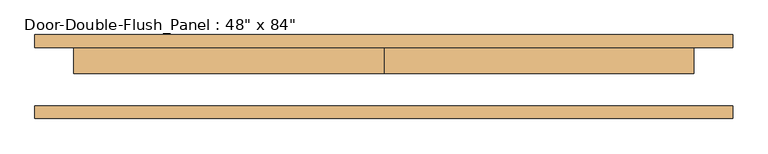
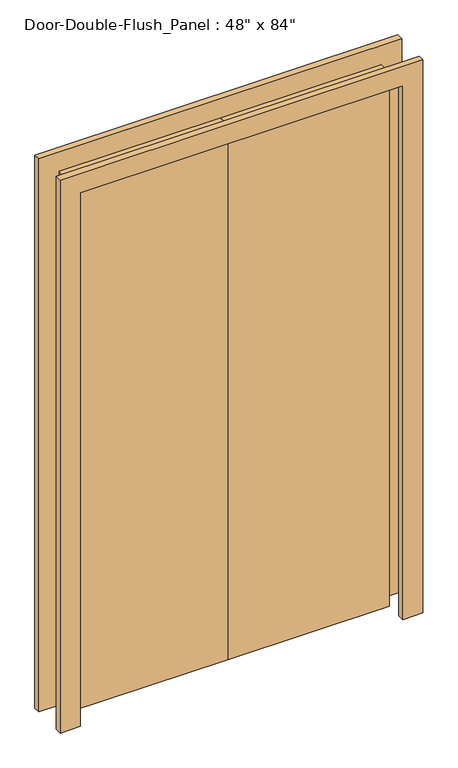
"""IFC4 building model written with IfcOpenShell, lengths in millimetres: door geometry."""

from ifc_helpers import new_model, si_unit, frame, origin, origin_with_axes, place, context, project, spatial, polyline, outline, extrude, source, transform, mapped, element, save


def door_eb8a45e1(model_context):
    return source(origin(), model_context, "Body", "SweptSolid", [
        extrude(outline(polyline([(2133.6, -609.6), (2133.6, 609.6), (0.0, 609.6), (0.0, 685.8), (2209.8, 685.8), (2209.8, -685.8), (0.0, -685.8), (0.0, -609.6), (2133.6, -609.6)])), frame((0.0, 57.15, 0.0), z_axis=(0.0, 1.0, 0.0), x_axis=(0.0, 0.0, 1.0)), (0.0, 0.0, 1.0), 25.4),
        extrude(outline(polyline([(2133.6, -609.6), (2133.6, 609.6), (0.0, 609.6), (0.0, 685.8), (2209.8, 685.8), (2209.8, -685.8), (0.0, -685.8), (0.0, -609.6), (2133.6, -609.6)])), frame((0.0, -82.55, 0.0), z_axis=(0.0, 1.0, 0.0), x_axis=(0.0, 0.0, 1.0)), (0.0, 0.0, 1.0), 25.4),
        extrude(outline(polyline([(-609.6, 57.15), (0.0, 57.15), (0.0, 6.35), (-609.6, 6.35), (-609.6, 57.15)])), origin_with_axes(), (0.0, 0.0, 1.0), 2133.6),
        extrude(outline(polyline([(0.0, 57.15), (609.6, 57.15), (609.6, 6.35), (0.0, 6.35), (0.0, 57.15)])), origin_with_axes(), (0.0, 0.0, 1.0), 2133.6),
    ])


if __name__ == "__main__":
    model = new_model("IFC4")
    model_context = context("Model", 3, world=origin())
    ifc_project = project(units=[si_unit("LENGTHUNIT", "METRE", prefix="MILLI")], contexts=[model_context])
    site = spatial("IfcSite", under=ifc_project)
    building = spatial("IfcBuilding", under=site)
    placement = place(None, origin())
    door_shape = door_eb8a45e1(model_context)
    element("IfcDoor", 1, ObjectType="Door-Double-Flush_Panel : 48\" x 84\"", at=placement, inside=building, context=model_context, shape_type="MappedRepresentation", body=[
        mapped(door_shape, transform((0.0, 0.0, 0.0), x_axis=(1.0, 0.0, 0.0), y_axis=(0.0, 1.0, 0.0), z_axis=(0.0, 0.0, 1.0))),
    ])
    save(model, "model.ifc")

# Revit data of these elements
# Type "Door-Double-Flush_Panel : 48\" x 84\""
#   Type Mark = "11"
#   Construction Type Id = "DOOR"
#   Assembly Code = "C1020"
#   Analytic Construction = "Wooden"
#   Thickness = 0' - 2"
#   Thermal Resistance (R) = 2.5876 (h·ft²·°F)/BTU
#   Swing Angle [instance default] = 90.00°
#   Panel Width = 2' - 0"
#   Heat Transfer Coefficient (U) = 0.3865 BTU/(h·ft²·°F)
#   Height = 7' - 0"
#   Trim Projection Ext = 0' - 1"
#   Trim Projection Int = 0' - 1"
#   Trim Width = 0' - 3"
#   Width = 4' - 0"
#   Define Thermal Properties by = 1
#   Panel Material = Wood - Birch - Solid Stained Light Low Gloss
#   Trim Material = Paint - Sienna
#   Visual Light Transmittance = 0
#   Solar Heat Gain Coefficient = 0
#   Function = (empty or 0)
#   Wall Closure = (empty or 0)
# Element 1 (IfcDoor, "Door-Double-Flush_Panel : 48\" x 84\"")
#   Materials on its faces: "Paint - Sienna", "Wood - Birch - Solid Stained Light Low Gloss"
# Materials
#   "Wood - Birch - Solid Stained Light Low Gloss": class "Wood", colour RGB 210 159 95, transparency 0, Cost = 0
#   "Paint - Sienna": colour RGB 118 70 51, transparency 0, Cost = 0
